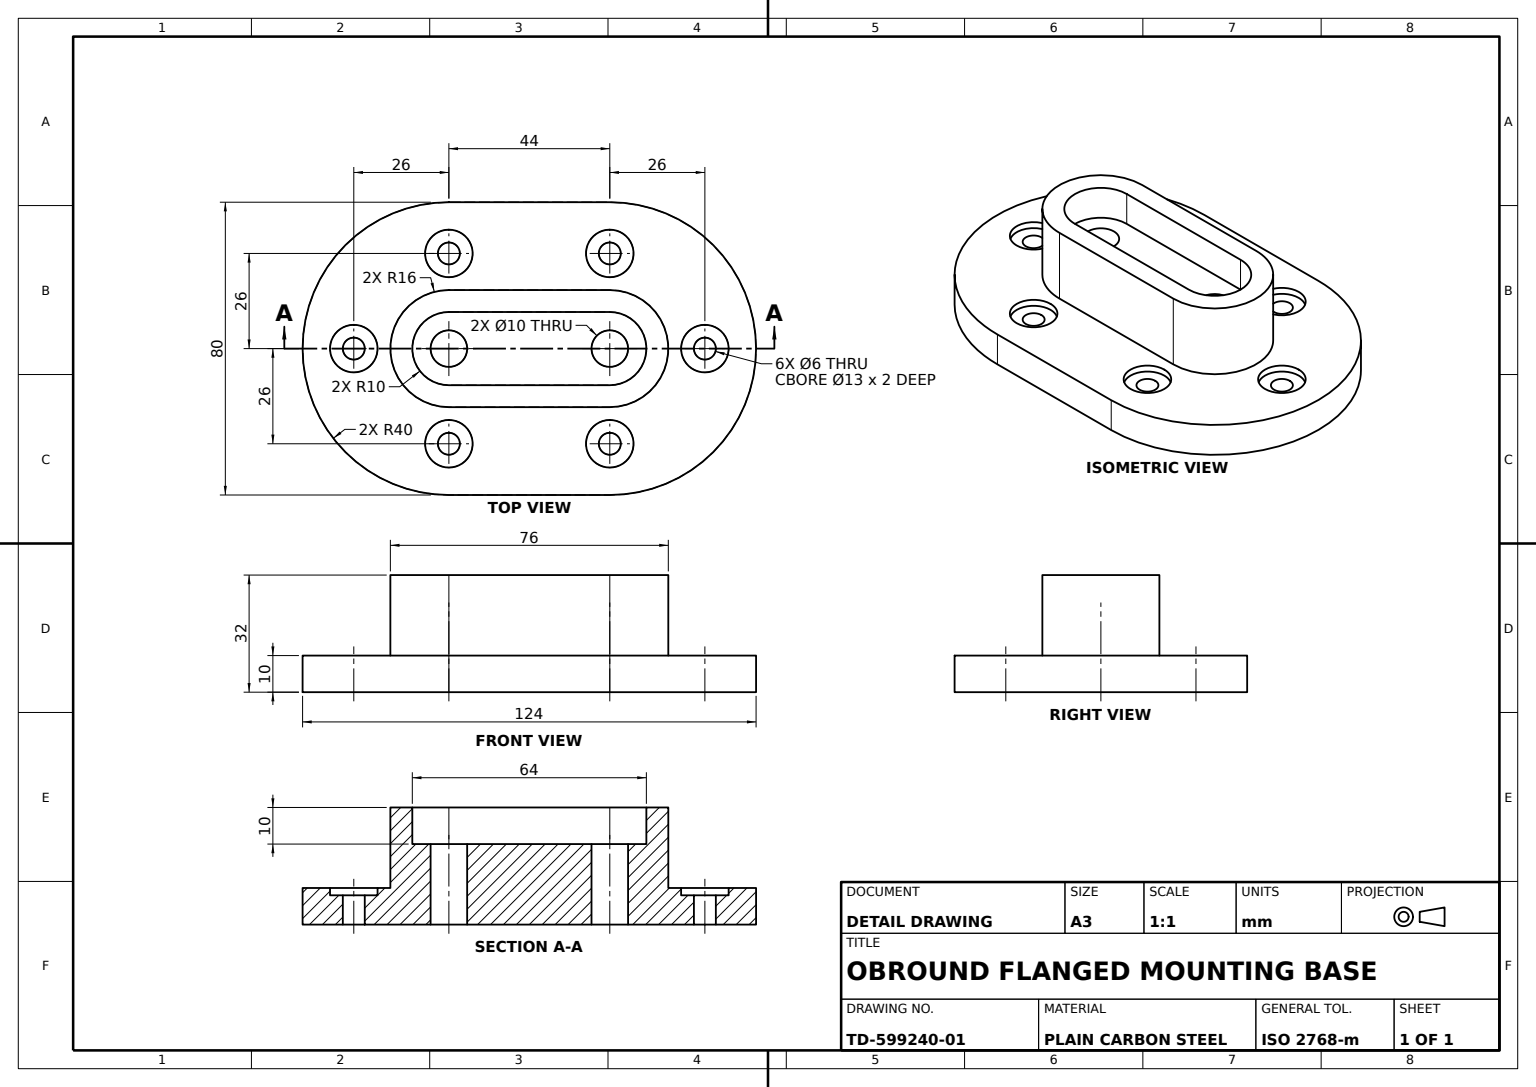
SolidWorks part; units mm, degrees
material "Plain Carbon Steel"
ref_plane "Front Plane" through (0, 0, 0) normal (0, 0, 1) x (1, 0, 0)
ref_plane "Top Plane" through (0, 0, 0) normal (0, 1, 0) x (1, 0, 0)
ref_plane "Right Plane" through (0, 0, 0) normal (1, 0, 0) x (0, 0, -1)
sketch "Base Flange Sketch" plane through (0, 0, 0) normal (0, 1, 0) x (1, 0, 0)
  line L0 (-22, -40) -> (22, -40)
  line L1 (-22, 40) -> (22, 40)
  arc A0 (22, -40) -> (22, 40) centre (22, 0) ccw
  arc A1 (-22, 40) -> (-22, -40) centre (-22, 0) ccw
  dimension "D1" = 40
  dimension "D2" = 44
  dimension "D3" = 22
extrude "Base Flange" add sketch "Base Flange Sketch" along normal blind 10
sketch "Slot Boss Sketch" plane through (0, 10, 0) normal (0, 1, 0) x (1, 0, 0)
  line L0 (-22, 16) -> (22, 16)
  line L1 (-22, -16) -> (22, -16)
  arc A0 (22, -16) -> (22, 16) centre (22, 0) ccw
  arc A1 (-22, 16) -> (-22, -16) centre (-22, 0) ccw
  dimension "D1" = 16
extrude "Slot Boss" add sketch "Slot Boss Sketch" along normal blind 22
sketch "Slot Pocket Sketch" plane through (0, 32, 0) normal (0, 1, 0) x (1, 0, 0)
  line L0 (-22, 10) -> (22, 10)
  line L1 (-22, -10) -> (22, -10)
  arc A0 (22, -10) -> (22, 10) centre (22, 0) ccw
  arc A1 (-22, 10) -> (-22, -10) centre (-22, 0) ccw
  dimension "D1" = 10
extrude "Slot Pocket" cut sketch "Slot Pocket Sketch" against normal blind 10
sketch "Slot Through Cut Sketch" plane through (0, 22, 0) normal (0, 1, 0) x (1, 0, 0)
  circle A0 centre (22, 0) radius 5
  circle A1 centre (-22, 0) radius 5
  dimension "D1" = 10
  dimension "D2" = 10
extrude "Slot Through Cut" cut sketch "Slot Through Cut Sketch" against normal blind 53
sketch "Counterbores Sketch" plane through (0, 10, 0) normal (0, 1, 0) x (1, 0, 0)
  circle A0 centre (48, 0) radius 6.5
  circle A1 centre (22, 26) radius 6.5
  circle A2 centre (-22, 26) radius 6.5
  circle A3 centre (-48, 0) radius 6.5
  circle A4 centre (-22, -26) radius 6.5
  circle A5 centre (22, -26) radius 6.5
  dimension "D1" = 13
  dimension "D2" = 13
  dimension "D3" = 13
  dimension "D4" = 13
  dimension "D5" = 13
  dimension "D6" = 13
  dimension "D7" = 22
  dimension "D8" = 26
  dimension "D9" = 48
  dimension "D10" = 22
  dimension "D11" = 48
  dimension "D12" = 22
  dimension "D13" = 26
  dimension "D14" = 26
  dimension "D15" = 22
  dimension "D16" = 26
extrude "Counterbores 6x Depth 2" cut sketch "Counterbores Sketch" against normal blind 2
sketch "Mounting Holes Sketch" plane through (0, 8, 0) normal (0, 1, 0) x (1, 0, 0)
  circle A0 centre (48, 0) radius 3
  circle A1 centre (22, -26) radius 3
  circle A2 centre (-22, -26) radius 3
  circle A3 centre (-48, 0) radius 3
  circle A4 centre (-22, 26) radius 3
  circle A5 centre (22, 26) radius 3
  dimension "D1" = 6
  dimension "D2" = 6
  dimension "D3" = 6
  dimension "D4" = 6
  dimension "D5" = 6
  dimension "D6" = 6
extrude "Mounting Holes 6x" cut sketch "Mounting Holes Sketch" against normal blind 40
